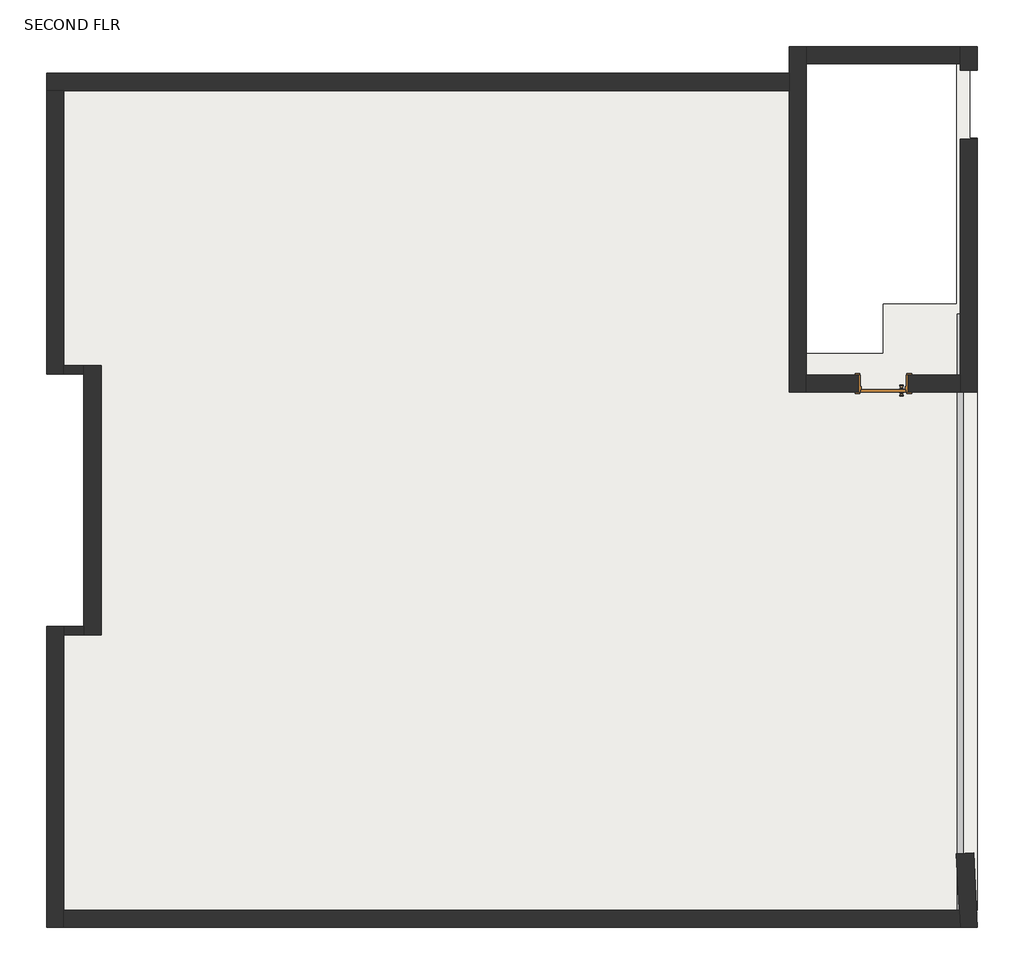
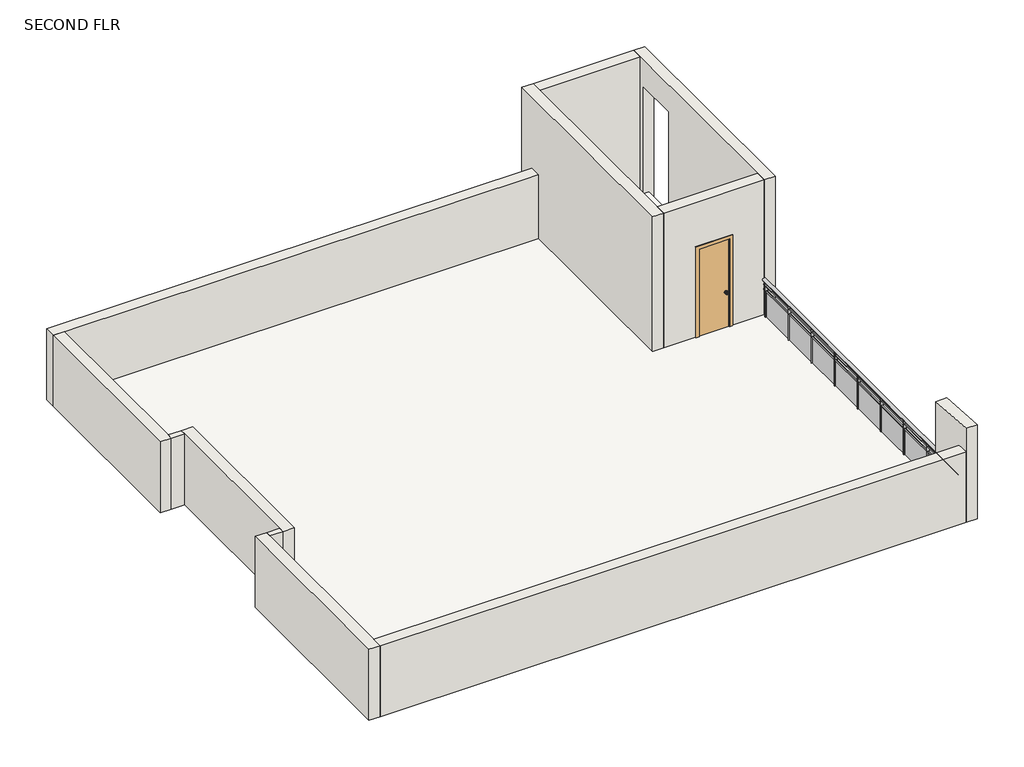
# One storey: 12 walls, 1 door, 1 railing, 1 roof.
"""IFC4 building model written with IfcOpenShell, lengths in millimetres."""

from ifc_helpers import new_model, si_unit, point, frame, origin, place, context, project, spatial, polyline, ellipse_curve, trimmed, outline, extrude, faceted_brep, transform, mapped, element, save
from ifc_brep_helpers import plane_surface, extruded_surface, advanced_brep
from components import door_bae2a1e9

model = new_model("IFC4")

# Units and contexts
model_context = context("Model", 3, world=origin())
ifc_project = project(units=[si_unit("LENGTHUNIT", "METRE", prefix="MILLI")], contexts=[model_context])

# Site, building, storey
site = spatial("IfcSite", under=ifc_project)
building = spatial("IfcBuilding", under=site)
storey = spatial("IfcBuildingStorey", under=building, Name="SECOND FLR", Elevation=6096.0)

# Door
placement = place(None, origin())
door_shape = door_bae2a1e9(model_context)
element("IfcDoor", 1, ObjectType="Door-Interior-Single-Flush_Panel-Wood : 24\" x 80\"", at=placement, inside=storey, context=model_context, shape_type="MappedRepresentation", body=[
    mapped(door_shape, transform((-3506.7156154, 2607.8968606, 6096.0), x_axis=(-1.0, 0.0, 0.0), y_axis=(0.0, -1.0, 0.0), z_axis=(0.0, 0.0, 1.0))),
])

# Railing
element("IfcRailing", 2, ObjectType="Glass Panel - Bottom Fill", at=placement, inside=storey, context=model_context, shape_type="SolidModel", body=[
    advanced_brep(
    [(-2522.4656154, -4390.5499125, 7010.4), (-2446.2656154, -4390.5499125, 7010.4), (-2522.4656154, 3534.2500875, 7010.4), (-2446.2656154, 3534.2500875, 7010.4)],
    [
        (0, 1, ellipse_curve(frame((-2484.3656154, -4390.5499125, 7010.4), z_axis=(0.0, -1.0, 0.0), x_axis=(1.0, 0.0, 0.0)), 38.1, 28.575)),
        (1, 0, ellipse_curve(frame((-2484.3656154, -4390.5499125, 7010.4), z_axis=(0.0, -1.0, 0.0), x_axis=(1.0, 0.0, 0.0)), 38.1, 28.575)),
        (2, 3, ellipse_curve(frame((-2484.3656154, 3534.2500875, 7010.4), z_axis=(0.0, 1.0, 0.0), x_axis=(1.0, 0.0, 0.0)), 38.1, 28.575)),
        (3, 2, ellipse_curve(frame((-2484.3656154, 3534.2500875, 7010.4), z_axis=(0.0, 1.0, 0.0), x_axis=(1.0, 0.0, 0.0)), 38.1, 28.575)),
        (0, 2),
        (3, 1),
    ],
    [
        plane_surface(frame((-2484.3656154, -4390.5499125, 7010.4), z_axis=(0.0, -1.0, 0.0), x_axis=(0.0, 0.0, 1.0))),
        plane_surface(frame((-2484.3656154, 3534.2500875, 7010.4), z_axis=(0.0, 1.0, 0.0), x_axis=(0.0, 0.0, 1.0))),
        extruded_surface(trimmed(ellipse_curve(frame((-2484.3656154, 3534.2500875, 7010.4), z_axis=(0.0, -1.0, 0.0), x_axis=(1.0, 0.0, 0.0)), 38.1, 28.575), [point((-2522.4656154, 3534.2500875, 7010.4))], [point((-2446.2656154, 3534.2500875, 7010.4))], True, "CARTESIAN"), (0.0, -7924.799999999999, 0.0), 7924.799999999999),
        extruded_surface(trimmed(ellipse_curve(frame((-2484.3656154, 3534.2500875, 7010.4), z_axis=(0.0, -1.0, 0.0), x_axis=(1.0, 0.0, 0.0)), 38.1, 28.575), [point((-2446.2656154, 3534.2500875, 7010.4))], [point((-2522.4656154, 3534.2500875, 7010.4))], True, "CARTESIAN"), (0.0, -7924.799999999999, 0.0), 7924.799999999999),
    ],
    [
        (0, [[1, 2]]),
        (1, [[3, 4]]),
        (2, [[-1, 5, -4, 6]]),
        (3, [[-2, -6, -3, -5]]),
    ],
),
    extrude(outline(polyline([(-2471.6656154, -4390.5499125), (-2497.0656154, -4390.5499125), (-2497.0656154, 3534.2500875), (-2471.6656154, 3534.2500875), (-2471.6656154, -4390.5499125)])), frame((0.0, 0.0, 6896.1), z_axis=(0.0, 0.0, 1.0), x_axis=(1.0, 0.0, 0.0)), (0.0, 0.0, 1.0), 25.4),
    extrude(outline(polyline([(-2471.6656154, -4390.5499125), (-2497.0656154, -4390.5499125), (-2497.0656154, 3534.2500875), (-2471.6656154, 3534.2500875), (-2471.6656154, -4390.5499125)])), frame((0.0, 0.0, 6794.5), z_axis=(0.0, 0.0, 1.0), x_axis=(1.0, 0.0, 0.0)), (0.0, 0.0, 1.0), 25.4),
    extrude(outline(polyline([(-2458.9656154, 3223.1000875), (-2509.7656154, 3223.1000875), (-2509.7656154, 3235.8000875), (-2458.9656154, 3235.8000875), (-2458.9656154, 3223.1000875)])), frame((0.0, 0.0, 6096.0), z_axis=(0.0, 0.0, 1.0), x_axis=(1.0, 0.0, 0.0)), (0.0, 0.0, 1.0), 885.825),
    extrude(outline(polyline([(-2490.9007724, 2416.6500875), (-2490.9007724, 3229.4500875), (-2484.5507724, 3229.4500875), (-2484.5507724, 2416.6500875), (-2490.9007724, 2416.6500875)])), frame((0.0, 0.0, 6197.6), z_axis=(0.0, 0.0, 1.0), x_axis=(1.0, 0.0, 0.0)), (0.0, 0.0, 1.0), 596.9),
    extrude(outline(polyline([(-2458.9656154, 2410.3000875), (-2509.7656154, 2410.3000875), (-2509.7656154, 2423.0000875), (-2458.9656154, 2423.0000875), (-2458.9656154, 2410.3000875)])), frame((0.0, 0.0, 6096.0), z_axis=(0.0, 0.0, 1.0), x_axis=(1.0, 0.0, 0.0)), (0.0, 0.0, 1.0), 885.825),
    extrude(outline(polyline([(-2490.9007724, 1603.8500875), (-2490.9007724, 2416.6500875), (-2484.5507724, 2416.6500875), (-2484.5507724, 1603.8500875), (-2490.9007724, 1603.8500875)])), frame((0.0, 0.0, 6197.6), z_axis=(0.0, 0.0, 1.0), x_axis=(1.0, 0.0, 0.0)), (0.0, 0.0, 1.0), 596.9),
    extrude(outline(polyline([(-2458.9656154, 1597.5000875), (-2509.7656154, 1597.5000875), (-2509.7656154, 1610.2000875), (-2458.9656154, 1610.2000875), (-2458.9656154, 1597.5000875)])), frame((0.0, 0.0, 6096.0), z_axis=(0.0, 0.0, 1.0), x_axis=(1.0, 0.0, 0.0)), (0.0, 0.0, 1.0), 885.825),
    extrude(outline(polyline([(-2490.9007724, 791.0500875), (-2490.9007724, 1603.8500875), (-2484.5507724, 1603.8500875), (-2484.5507724, 791.0500875), (-2490.9007724, 791.0500875)])), frame((0.0, 0.0, 6197.6), z_axis=(0.0, 0.0, 1.0), x_axis=(1.0, 0.0, 0.0)), (0.0, 0.0, 1.0), 596.9),
    extrude(outline(polyline([(-2458.9656154, 784.7000875), (-2509.7656154, 784.7000875), (-2509.7656154, 797.4000875), (-2458.9656154, 797.4000875), (-2458.9656154, 784.7000875)])), frame((0.0, 0.0, 6096.0), z_axis=(0.0, 0.0, 1.0), x_axis=(1.0, 0.0, 0.0)), (0.0, 0.0, 1.0), 885.825),
    extrude(outline(polyline([(-2490.9007724, -21.7499125), (-2490.9007724, 791.0500875), (-2484.5507724, 791.0500875), (-2484.5507724, -21.7499125), (-2490.9007724, -21.7499125)])), frame((0.0, 0.0, 6197.6), z_axis=(0.0, 0.0, 1.0), x_axis=(1.0, 0.0, 0.0)), (0.0, 0.0, 1.0), 596.9),
    extrude(outline(polyline([(-2458.9656154, -28.0999125), (-2509.7656154, -28.0999125), (-2509.7656154, -15.3999125), (-2458.9656154, -15.3999125), (-2458.9656154, -28.0999125)])), frame((0.0, 0.0, 6096.0), z_axis=(0.0, 0.0, 1.0), x_axis=(1.0, 0.0, 0.0)), (0.0, 0.0, 1.0), 885.825),
    extrude(outline(polyline([(-2490.9007724, -834.5499125), (-2490.9007724, -21.7499125), (-2484.5507724, -21.7499125), (-2484.5507724, -834.5499125), (-2490.9007724, -834.5499125)])), frame((0.0, 0.0, 6197.6), z_axis=(0.0, 0.0, 1.0), x_axis=(1.0, 0.0, 0.0)), (0.0, 0.0, 1.0), 596.9),
    extrude(outline(polyline([(-2458.9656154, -840.8999125), (-2509.7656154, -840.8999125), (-2509.7656154, -828.1999125), (-2458.9656154, -828.1999125), (-2458.9656154, -840.8999125)])), frame((0.0, 0.0, 6096.0), z_axis=(0.0, 0.0, 1.0), x_axis=(1.0, 0.0, 0.0)), (0.0, 0.0, 1.0), 885.825),
    extrude(outline(polyline([(-2490.9007724, -1647.3499125), (-2490.9007724, -834.5499125), (-2484.5507724, -834.5499125), (-2484.5507724, -1647.3499125), (-2490.9007724, -1647.3499125)])), frame((0.0, 0.0, 6197.6), z_axis=(0.0, 0.0, 1.0), x_axis=(1.0, 0.0, 0.0)), (0.0, 0.0, 1.0), 596.9),
    extrude(outline(polyline([(-2458.9656154, -1653.6999125), (-2509.7656154, -1653.6999125), (-2509.7656154, -1640.9999125), (-2458.9656154, -1640.9999125), (-2458.9656154, -1653.6999125)])), frame((0.0, 0.0, 6096.0), z_axis=(0.0, 0.0, 1.0), x_axis=(1.0, 0.0, 0.0)), (0.0, 0.0, 1.0), 885.825),
    extrude(outline(polyline([(-2490.9007724, -2460.1499125), (-2490.9007724, -1647.3499125), (-2484.5507724, -1647.3499125), (-2484.5507724, -2460.1499125), (-2490.9007724, -2460.1499125)])), frame((0.0, 0.0, 6197.6), z_axis=(0.0, 0.0, 1.0), x_axis=(1.0, 0.0, 0.0)), (0.0, 0.0, 1.0), 596.9),
    extrude(outline(polyline([(-2458.9656154, -2466.4999125), (-2509.7656154, -2466.4999125), (-2509.7656154, -2453.7999125), (-2458.9656154, -2453.7999125), (-2458.9656154, -2466.4999125)])), frame((0.0, 0.0, 6096.0), z_axis=(0.0, 0.0, 1.0), x_axis=(1.0, 0.0, 0.0)), (0.0, 0.0, 1.0), 885.825),
    extrude(outline(polyline([(-2490.9007724, -3272.9499125), (-2490.9007724, -2460.1499125), (-2484.5507724, -2460.1499125), (-2484.5507724, -3272.9499125), (-2490.9007724, -3272.9499125)])), frame((0.0, 0.0, 6197.6), z_axis=(0.0, 0.0, 1.0), x_axis=(1.0, 0.0, 0.0)), (0.0, 0.0, 1.0), 596.9),
    extrude(outline(polyline([(-2458.9656154, -3279.2999125), (-2509.7656154, -3279.2999125), (-2509.7656154, -3266.5999125), (-2458.9656154, -3266.5999125), (-2458.9656154, -3279.2999125)])), frame((0.0, 0.0, 6096.0), z_axis=(0.0, 0.0, 1.0), x_axis=(1.0, 0.0, 0.0)), (0.0, 0.0, 1.0), 885.825),
    extrude(outline(polyline([(-2490.9007724, -4085.7499125), (-2490.9007724, -3272.9499125), (-2484.5507724, -3272.9499125), (-2484.5507724, -4085.7499125), (-2490.9007724, -4085.7499125)])), frame((0.0, 0.0, 6197.6), z_axis=(0.0, 0.0, 1.0), x_axis=(1.0, 0.0, 0.0)), (0.0, 0.0, 1.0), 596.9),
    extrude(outline(polyline([(-2458.9656154, -4092.0999125), (-2509.7656154, -4092.0999125), (-2509.7656154, -4079.3999125), (-2458.9656154, -4079.3999125), (-2458.9656154, -4092.0999125)])), frame((0.0, 0.0, 6096.0), z_axis=(0.0, 0.0, 1.0), x_axis=(1.0, 0.0, 0.0)), (0.0, 0.0, 1.0), 885.825),
    extrude(outline(polyline([(-2474.8406154, 3521.5500875), (-2493.8906154, 3521.5500875), (-2493.8906154, 3540.6000875), (-2474.8406154, 3540.6000875), (-2474.8406154, 3521.5500875)])), frame((0.0, 0.0, 6096.0), z_axis=(0.0, 0.0, 1.0), x_axis=(1.0, 0.0, 0.0)), (0.0, 0.0, 1.0), 885.825),
    extrude(outline(polyline([(-2474.8406154, -4396.8999125), (-2493.8906154, -4396.8999125), (-2493.8906154, -4377.8499125), (-2474.8406154, -4377.8499125), (-2474.8406154, -4396.8999125)])), frame((0.0, 0.0, 6096.0), z_axis=(0.0, 0.0, 1.0), x_axis=(1.0, 0.0, 0.0)), (0.0, 0.0, 1.0), 885.825),
])

# Roof
element("IfcRoof", 3, ObjectType="roof material", at=placement, inside=storey, context=model_context, shape_type="Brep", body=[
    faceted_brep([(-14396.9656154, 6506.0500875, 6096.0), (-4757.6656154, 6506.0500875, 6096.0), (-4757.6656154, 7090.2500875, 6096.0), (-2357.3656154, 7090.2500875, 6096.0), (-2357.3656154, 6772.7500875, 6096.0), (-2357.3656154, 6125.0500875, 6096.0), (-2357.3656154, 5871.0500875, 6096.0), (-2255.7656154, 5871.0500875, 6096.0), (-2255.7656154, -4393.7249125, 6096.0), (-14396.9656154, -4393.7249125, 6096.0), (-14396.9656154, -618.6499125, 6096.0), (-13901.6656154, -618.6499125, 6096.0), (-13901.6656154, 2848.4500875, 6096.0), (-14396.9656154, 2848.4500875, 6096.0), (-2535.1656154, 3672.7728408, 6096.0), (-2535.1656154, 6861.6500875, 6096.0), (-4529.0656154, 6861.6500875, 6096.0), (-4529.0656154, 3672.7728408, 6096.0), (-4529.0656154, 3012.3728408, 6096.0), (-3513.0656154, 3012.3728408, 6096.0), (-3513.0656154, 3672.7728408, 6096.0), (-4757.6656154, 6506.0500875, 6248.4), (-14396.9656154, 6506.0500875, 6248.4), (-14396.9656154, 2848.4500875, 6248.4), (-13901.6656154, 2848.4500875, 6248.4), (-13901.6656154, -618.6499125, 6248.4), (-14396.9656154, -618.6499125, 6248.4), (-14396.9656154, -4393.7249125, 6248.4), (-2255.7656154, -4393.7249125, 6248.4), (-2255.7656154, 2496.7718606, 6248.4), (-2255.7656154, 5858.3500875, 6248.4), (-2255.7656154, 5871.0500875, 6248.4), (-2357.3656154, 5871.0500875, 6248.4), (-2357.3656154, 6125.0500875, 6248.4), (-2357.3656154, 6772.7500875, 6248.4), (-2357.3656154, 7090.2500875, 6248.4), (-2484.3656154, 7090.2500875, 6248.4), (-4757.6656154, 7090.2500875, 6248.4), (-2535.1656154, 6861.6500875, 6248.4), (-2535.1656154, 3672.7728408, 6248.4), (-3513.0656154, 3672.7728408, 6248.4), (-3513.0656154, 3012.3728408, 6248.4), (-4529.0656154, 3012.3728408, 6248.4), (-4529.0656154, 3672.7728408, 6248.4), (-4529.0656154, 6861.6500875, 6248.4)], [[[0, 1, 2, 3, 4, 5, 6, 7, 8, 9, 10, 11, 12, 13], [14, 15, 16, 17, 18, 19, 20]], [[21, 22, 23, 24, 25, 26, 27, 28, 29, 30, 31, 32, 33, 34, 35, 36, 37], [38, 39, 40, 41, 42, 43, 44]], [[1, 0, 22, 21]], [[2, 1, 21, 37]], [[3, 2, 37, 36, 35]], [[9, 8, 28, 27]], [[8, 7, 31, 30, 29, 28]], [[0, 13, 23, 22]], [[10, 9, 27, 26]], [[38, 15, 14, 39]], [[39, 14, 20, 40]], [[40, 20, 19, 41]], [[41, 19, 18, 42]], [[42, 18, 17, 43]], [[43, 17, 16, 44]], [[15, 38, 44, 16]], [[5, 4, 3, 35, 34, 33]], [[7, 6, 32, 31]], [[6, 5, 33, 32]], [[13, 12, 24, 23]], [[12, 11, 25, 24]], [[11, 10, 26, 25]]]),
])

# Walls
element("IfcWall", 4, at=placement, inside=storey, context=model_context, shape_type="Brep", body=[
    faceted_brep([(-2484.3656154, 2496.7718606, 9144.0), (-2484.3656154, 2725.3718606, 9144.0), (-2484.3656154, 6861.6500875, 9144.0), (-2484.3656154, 7090.2500875, 9144.0), (-2484.3656154, 7090.2500875, 6248.4), (-2484.3656154, 6772.7500875, 6248.4), (-2484.3656154, 6772.7500875, 8564.5201514), (-2484.3656154, 5858.3500875, 8564.5201514), (-2484.3656154, 5858.3500875, 6248.4), (-2484.3656154, 2496.7718606, 6248.4), (-2255.7656154, 7090.2500875, 9144.0), (-2255.7656154, 2496.7718606, 9144.0), (-2255.7656154, 2496.7718606, 6248.4), (-2255.7656154, 5858.3500875, 6248.4), (-2255.7656154, 5858.3500875, 8564.5201514), (-2255.7656154, 6772.7500875, 8564.5201514), (-2255.7656154, 6772.7500875, 6096.0), (-2255.7656154, 7090.2500875, 6096.0), (-2357.3656154, 6772.7500875, 6096.0), (-2357.3656154, 7090.2500875, 6096.0), (-2357.3656154, 7090.2500875, 6248.4), (-2357.3656154, 6772.7500875, 6248.4)], [[[0, 1, 2, 3, 4, 5, 6, 7, 8, 9]], [[10, 11, 12, 13, 14, 15, 16, 17]], [[17, 16, 18, 19]], [[3, 2, 1, 0, 11, 10]], [[3, 10, 17, 19, 20, 4]], [[9, 8, 13, 12]], [[20, 21, 5, 4]], [[11, 0, 9, 12]], [[15, 6, 5, 21, 18, 16]], [[6, 15, 14, 7]], [[7, 14, 13, 8]], [[21, 20, 19, 18]]]),
])
element("IfcWall", 5, at=placement, inside=storey, context=model_context, shape_type="Brep", body=[
    faceted_brep([(-4529.0656154, 2496.7718606, 6096.0), (-4529.0656154, 2725.3718606, 6096.0), (-4529.0656154, 6861.6500875, 6096.0), (-4529.0656154, 7090.2500875, 6096.0), (-4529.0656154, 7090.2500875, 9144.0), (-4529.0656154, 6861.6500875, 9144.0), (-4529.0656154, 2725.3718606, 9144.0), (-4529.0656154, 2496.7718606, 9144.0), (-4757.6656154, 2496.7718606, 6096.0), (-4757.6656154, 2496.7718606, 9144.0), (-4757.6656154, 7090.2500875, 9144.0), (-4757.6656154, 7090.2500875, 6096.0), (-4757.6656154, 6734.6500875, 6096.0), (-4757.6656154, 6506.0500875, 6096.0)], [[[0, 1, 2, 3, 4, 5, 6, 7]], [[8, 9, 10, 11, 12, 13]], [[3, 2, 1, 0, 8, 13, 12, 11]], [[7, 6, 5, 4, 10, 9]], [[4, 3, 11, 10]], [[0, 7, 9, 8]]]),
])
element("IfcWall", 6, at=placement, inside=storey, context=model_context, shape_type="Brep", body=[
    faceted_brep([(-4529.0656154, 6861.6500875, 6096.0), (-2484.3656154, 6861.6500875, 6096.0), (-2484.3656154, 6861.6500875, 9144.0), (-4529.0656154, 6861.6500875, 9144.0), (-4529.0656154, 7090.2500875, 6096.0), (-4529.0656154, 7090.2500875, 9144.0), (-2484.3656154, 7090.2500875, 9144.0), (-2484.3656154, 7090.2500875, 6248.4), (-2484.3656154, 7090.2500875, 6096.0)], [[[0, 1, 2, 3]], [[4, 5, 6, 7, 8]], [[1, 0, 4, 8]], [[3, 2, 6, 5]], [[0, 3, 5, 4]], [[2, 1, 8, 7, 6]]]),
])
element("IfcWall", 7, at=placement, inside=storey, context=model_context, shape_type="Brep", body=[
    faceted_brep([(-2255.7656154, -4619.1499125, 6096.0), (-2307.6096137, -3629.9074953, 6096.0), (-2307.6096137, -3629.9074953, 8119.2878213), (-2255.7656154, -4619.1499125, 8119.2878213), (-2484.6793337, -4619.1499125, 6096.0), (-2484.6793337, -4619.1499125, 7620.0), (-2484.6793337, -4619.1499125, 8119.2878213), (-2535.8963253, -3641.8714949, 8119.2878213), (-2535.8963253, -3641.8714949, 6096.0), (-2496.6597521, -4390.5499125, 6096.0)], [[[0, 1, 2, 3]], [[4, 5, 6, 7, 8, 9]], [[1, 0, 4, 9, 8]], [[2, 1, 8, 7]], [[3, 2, 7, 6]], [[0, 3, 6, 5, 4]]]),
])
element("IfcWall", 8, at=placement, inside=storey, context=model_context, shape_type="Brep", body=[
    faceted_brep([(-4529.0656154, 2725.3718606, 9144.0), (-2484.3656154, 2725.3718606, 9144.0), (-2484.3656154, 2725.3718606, 6096.0), (-3176.5156154, 2725.3718606, 6096.0), (-3176.5156154, 2725.3718606, 8153.4), (-3836.9156154, 2725.3718606, 8153.4), (-3836.9156154, 2725.3718606, 6096.0), (-4529.0656154, 2725.3718606, 6096.0), (-2484.3656154, 2496.7718606, 9144.0), (-4529.0656154, 2496.7718606, 9144.0), (-4529.0656154, 2496.7718606, 6096.0), (-3836.9156154, 2496.7718606, 6096.0), (-3836.9156154, 2496.7718606, 8153.4), (-3176.5156154, 2496.7718606, 8153.4), (-3176.5156154, 2496.7718606, 6096.0), (-2484.3656154, 2496.7718606, 6096.0), (-2484.3656154, 2496.7718606, 6248.4)], [[[0, 1, 2, 3, 4, 5, 6, 7]], [[8, 9, 10, 11, 12, 13, 14, 15, 16]], [[2, 15, 14, 3]], [[10, 7, 6, 11]], [[1, 0, 9, 8]], [[2, 1, 8, 16, 15]], [[0, 7, 10, 9]], [[5, 12, 11, 6]], [[12, 5, 4, 13]], [[13, 4, 3, 14]]]),
])
element("IfcWall", 9, at=placement, inside=storey, context=model_context, shape_type="Brep", body=[
    faceted_brep([(-4757.6656154, 6734.6500875, 6096.0), (-14625.5656154, 6734.6500875, 6096.0), (-14625.5656154, 6734.6500875, 7620.0), (-4757.6656154, 6734.6500875, 7620.0), (-4757.6656154, 6506.0500875, 6096.0), (-4757.6656154, 6506.0500875, 7620.0), (-14396.9656154, 6506.0500875, 7620.0), (-14625.5656154, 6506.0500875, 7620.0), (-14625.5656154, 6506.0500875, 6096.0), (-14396.9656154, 6506.0500875, 6096.0)], [[[0, 1, 2, 3]], [[4, 5, 6, 7, 8, 9]], [[1, 0, 4, 9, 8]], [[3, 2, 7, 6, 5]], [[0, 3, 5, 4]], [[2, 1, 8, 7]]]),
])
element("IfcWall", 10, at=placement, inside=storey, context=model_context, shape_type="Brep", body=[
    faceted_brep([(-14625.5656154, 6506.0500875, 6096.0), (-14625.5656154, 2734.1500875, 6096.0), (-14625.5656154, 2734.1500875, 7620.0), (-14625.5656154, 6506.0500875, 7620.0), (-14396.9656154, 6506.0500875, 6096.0), (-14396.9656154, 6506.0500875, 7620.0), (-14396.9656154, 2848.4500875, 7620.0), (-14396.9656154, 2734.1500875, 7620.0), (-14396.9656154, 2734.1500875, 6096.0), (-14396.9656154, 2848.4500875, 6096.0)], [[[0, 1, 2, 3]], [[4, 5, 6, 7, 8, 9]], [[1, 0, 4, 9, 8]], [[3, 2, 7, 6, 5]], [[0, 3, 5, 4]], [[2, 1, 8, 7]]]),
])
element("IfcWall", 11, at=placement, inside=storey, context=model_context, shape_type="Brep", body=[
    faceted_brep([(-14130.2656154, 2848.4500875, 6096.0), (-14130.2656154, 2734.1500875, 6096.0), (-14130.2656154, -618.6499125, 6096.0), (-14130.2656154, -732.9499125, 6096.0), (-14130.2656154, -732.9499125, 7620.0), (-14130.2656154, -618.6499125, 7620.0), (-14130.2656154, 2734.1500875, 7620.0), (-14130.2656154, 2848.4500875, 7620.0), (-13901.6656154, 2848.4500875, 6096.0), (-13901.6656154, 2848.4500875, 7620.0), (-13901.6656154, -732.9499125, 7620.0), (-13901.6656154, -732.9499125, 6096.0)], [[[0, 1, 2, 3, 4, 5, 6, 7]], [[8, 9, 10, 11]], [[3, 2, 1, 0, 8, 11]], [[7, 6, 5, 4, 10, 9]], [[0, 7, 9, 8]], [[4, 3, 11, 10]]]),
])
element("IfcWall", 12, at=placement, inside=storey, context=model_context, shape_type="Brep", body=[
    faceted_brep([(-14625.5656154, -618.6499125, 6096.0), (-14625.5656154, -4619.1499125, 6096.0), (-14625.5656154, -4619.1499125, 7620.0), (-14625.5656154, -618.6499125, 7620.0), (-14396.9656154, -618.6499125, 6096.0), (-14396.9656154, -618.6499125, 7620.0), (-14396.9656154, -732.9499125, 7620.0), (-14396.9656154, -4390.5499125, 7620.0), (-14396.9656154, -4619.1499125, 7620.0), (-14396.9656154, -4619.1499125, 6096.0), (-14396.9656154, -4390.5499125, 6096.0), (-14396.9656154, -732.9499125, 6096.0)], [[[0, 1, 2, 3]], [[4, 5, 6, 7, 8, 9, 10, 11]], [[1, 0, 4, 11, 10, 9]], [[3, 2, 8, 7, 6, 5]], [[2, 1, 9, 8]], [[0, 3, 5, 4]]]),
])
element("IfcWall", 13, at=placement, inside=storey, context=model_context, shape_type="SweptSolid", body=[
    extrude(outline(polyline([(-2484.6793337, -4619.1499125), (-14396.9656154, -4619.1499125), (-14396.9656154, -4390.5499125), (-2496.6597521, -4390.5499125), (-2484.6793337, -4619.1499125)])), frame((0.0, 0.0, 6096.0), z_axis=(0.0, 0.0, 1.0), x_axis=(1.0, 0.0, 0.0)), (0.0, 0.0, 1.0), 1524.0),
])
element("IfcWall", 14, at=placement, inside=storey, context=model_context, shape_type="SweptSolid", body=[
    extrude(outline(polyline([(-14130.2656154, 2734.1500875), (-14396.9656154, 2734.1500875), (-14396.9656154, 2848.4500875), (-14130.2656154, 2848.4500875), (-14130.2656154, 2734.1500875)])), frame((0.0, 0.0, 6096.0), z_axis=(0.0, 0.0, 1.0), x_axis=(1.0, 0.0, 0.0)), (0.0, 0.0, 1.0), 1524.0),
])
element("IfcWall", 15, at=placement, inside=storey, context=model_context, shape_type="SweptSolid", body=[
    extrude(outline(polyline([(-14130.2656154, -732.9499125), (-14396.9656154, -732.9499125), (-14396.9656154, -618.6499125), (-14130.2656154, -618.6499125), (-14130.2656154, -732.9499125)])), frame((0.0, 0.0, 6096.0), z_axis=(0.0, 0.0, 1.0), x_axis=(1.0, 0.0, 0.0)), (0.0, 0.0, 1.0), 1524.0),
])

save(model, "model.ifc")

# Revit data of these elements
# Type "Door-Interior-Single-Flush_Panel-Wood : 24\" x 80\""
#   Type Mark = "12"
#   Assembly Code = "C1020300"
#   Analytic Construction = "Wooden"
#   Thickness = 0' - 1 3/8"
#   Thermal Resistance (R) = 2.5876 (h·ft²·°F)/BTU
#   Swing Angle [instance default] = 90.00°
#   Rough Width = 2' - 2"
#   Rough Height = 6' - 9"
#   Height = 6' - 8"
#   Width = 2' - 0"
#   Heat Transfer Coefficient (U) = 0.3865 BTU/(h·ft²·°F)
#   Trim Material = Cherry
#   Panel Material = Cherry
#   Frame Material = Cherry
#   Door Handle Material = Aluminum
#   Visual Light Transmittance = 0
#   Solar Heat Gain Coefficient = 0
#   Wall Closure = (empty or 0)
#   Function = (empty or 0)
# Type "Glass Panel - Bottom Fill"
#   Assembly Code = "C2010400"
#   built-in parameter 1008612 = 0.0416667 (stored number, unit not read)
#   built-in parameter 1008611 = 0.0416667 (stored number, unit not read)
#   built-in parameter 1008609 = 0.333333 (stored number, unit not read)
#   built-in parameter 1008604 = 0.166667 (stored number, unit not read)
#   built-in parameter 1008603 = 0.166667 (stored number, unit not read)
#   Railing Height = 3' - 0"
#   built-in parameter 1008630 = 2
#   built-in parameter 1008610 = 2
#   built-in parameter 1008618 = Baluster - Square : 3/4"
# Type "roof material"
#   Assembly Code = "B1020"
#   Layers, outside or top first: 0' - 6" "roof material" (function 1)
# Type
#   Assembly Code = "B2010"
#   Layers, outside or top first: 0' - 9" "LIGHT BEIGE" (function 1)
# Type
#   Assembly Code = "B2010"
#   Layers, outside or top first: 0' - 4 1/2" "LIGHT BEIGE" (function 1)
# Element 1 (IfcDoor, "Door-Interior-Single-Flush_Panel-Wood : 24\" x 80\"")
#   Swing Angle = 90.00°
#   Phase Created = New Construction
#   Materials on its faces: "Cherry", "Aluminum"
# Element 2 (IfcRailing, "Glass Panel - Bottom Fill")
#   Phase Created = New Construction
#   Materials on its faces: "Glass"
# Element 3 (IfcRoof, "roof material")
#   built-in parameter 1001705 = 20.5 (stored number, unit not read)
#   built-in parameter 1001710 = 33615
#   Phase Created = New Construction
#   Materials on its faces: "roof material"
# Elements 4, 5, 6, 8 (IfcWall)
#   Top Offset = 0' - 0"
#   Base Offset = 0' - 0"
#   wall height = 10' - 0"
#   Phase Created = New Construction
#   Base Constraint = SECOND FLR
#   Top Constraint = TOP OF ROOF
#   Materials on its faces: "LIGHT BEIGE"
# Element 7 (IfcWall)
#   Top Offset = -3' - 4.343"
#   Base Offset = 0' - 0"
#   wall height = 6' - 7.657"
#   Phase Created = New Construction
#   Base Constraint = SECOND FLR
#   Top Constraint = TOP OF ROOF
#   Materials on its faces: "LIGHT BEIGE", "Concrete, Cast-in-Place gray"
# Elements 9, 10, 11, 12, 13, 14, 15 (IfcWall)
#   Top Offset = 0' - 0"
#   Base Offset = 0' - 0"
#   Unconnected Height = 5' - 0"
#   wall height = 5' - 0"
#   Phase Created = New Construction
#   Base Constraint = SECOND FLR
#   Materials on its faces: "LIGHT BEIGE"
# Materials
#   "Cherry": class "Wood", colour RGB 226 177 128, transparency 0, Description = "Prunus Serotina", Cost = 0
#   "Aluminum": class "Metal", colour RGB 247 247 247, transparency 0, Description = "Aluminum 6061", Cost = 0
#   "roof material": class "Generic", colour RGB 120 120 120, transparency 0, Cost = 0
#   "LIGHT BEIGE": class "Generic", colour RGB 120 120 120, transparency 0, Cost = 0
#   "Glass": class "Glass", colour RGB 0 128 192, transparency 0.75, Description = "Soda Lime Glass", Cost = 0
#   "Concrete, Cast-in-Place gray": class "Concrete", colour RGB 192 192 192, transparency 0, Description = "Cast-in-place concrete", Cost = 0
